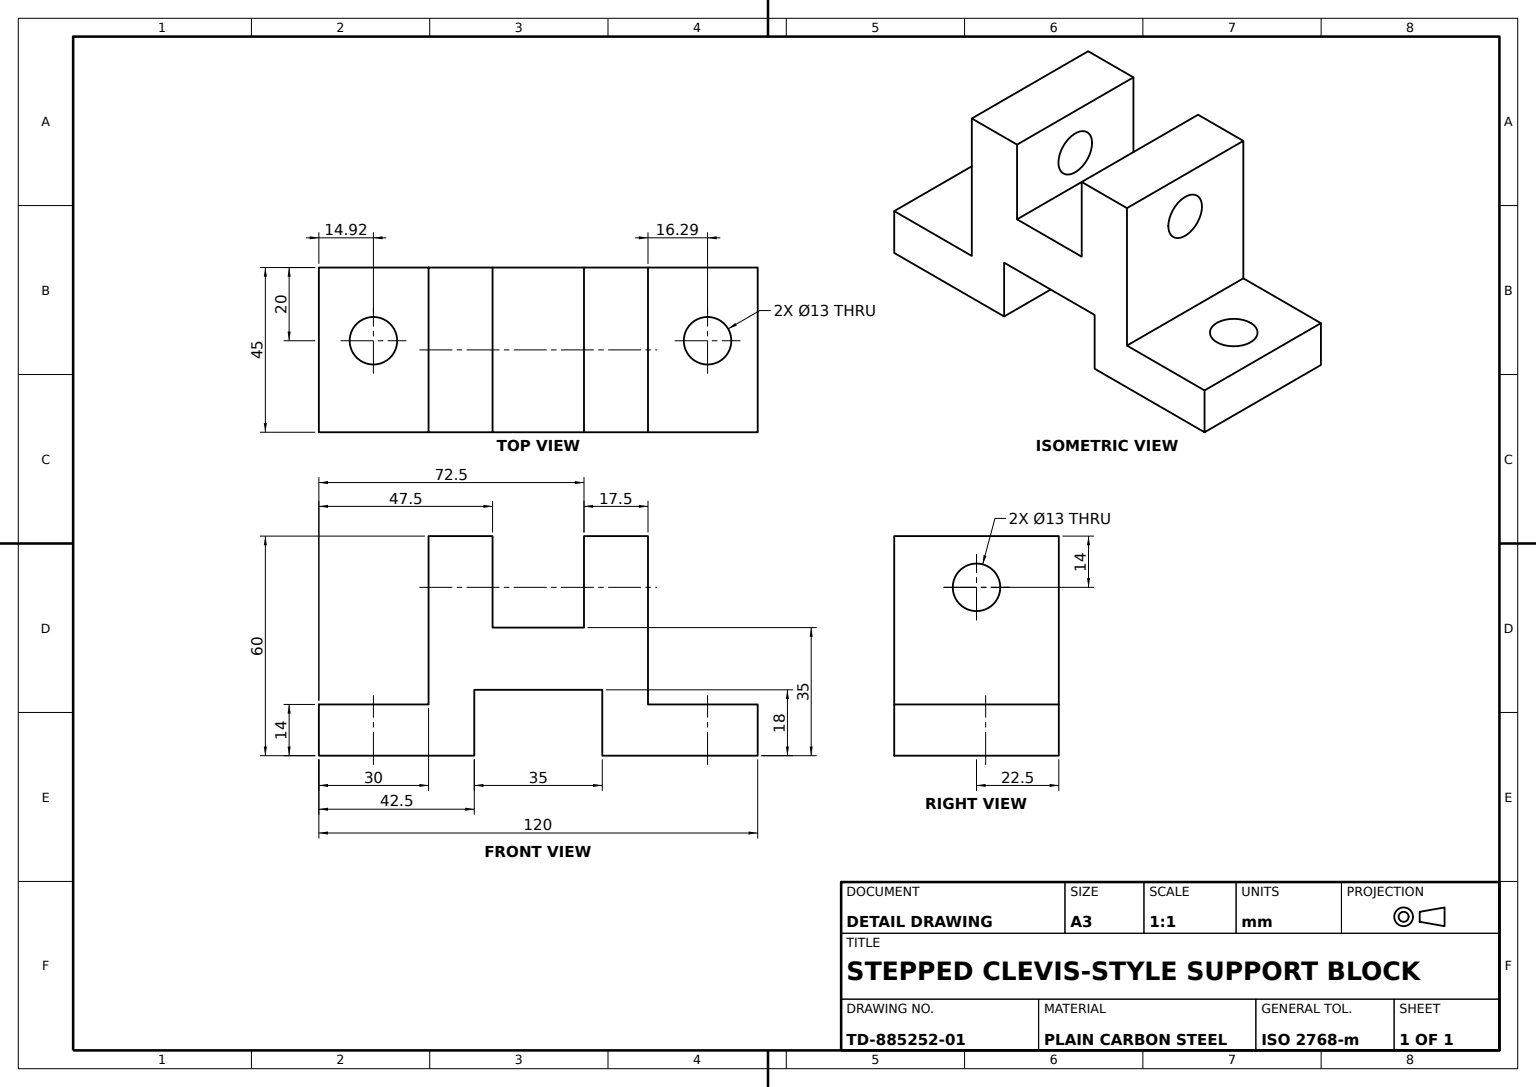
from build123d import *

# Parameters (mm, degrees)
BRACKET_BODY_DEPTH      = 45
UPRIGHT_HOLE_A_SKETCH_R = 6.5
UPRIGHT_HOLE_A_13_DEPTH = 17.5
UPRIGHT_START           = -17.5
UPRIGHT_HOLE_B_SKETCH_R = 6.5
UPRIGHT_HOLE_B_13_DEPTH = 17.5
FLANGE_HOLE_A_SKETCH_R  = 6.5
FLANGE_HOLE_A_13_DEPTH  = 14
FLANGE_HOLE_B_SKETCH_R  = 6.5
FLANGE_HOLE_B_13_DEPTH  = 14


with BuildPart() as part:
    # Bracket Profile Sketch → Bracket Body (new body)
    with BuildSketch(Plane.XY):
        Polygon((0, 0), (42.5, 0), (42.5, 18), (77.5, 18), (77.5, 0), (120, 0), (120, 14), (90, 14), (90, 60), (72.5, 60), (72.5, 35), (47.5, 35), (47.5, 60), (30, 60), (30, 14), (0, 14), align=None)
    extrude(amount=BRACKET_BODY_DEPTH)

    # Upright Hole A Sketch → Upright Hole A Ø13 (cut)
    with BuildSketch(Plane.ZY.offset(-30)):
        with Locations((22.5, 46)):
            Circle(UPRIGHT_HOLE_A_SKETCH_R)
    extrude(amount=-UPRIGHT_HOLE_A_13_DEPTH, mode=Mode.SUBTRACT)

    # Upright Hole B Sketch → Upright Hole B Ø13 (cut)
    with BuildSketch(Plane(origin=(90, 0, 0), x_dir=(0, 0, -1), z_dir=(1, 0, 0)).offset(UPRIGHT_START)):
        with Locations(Location((-22.5, 46, 0), (0, 0, 180))):
            Circle(UPRIGHT_HOLE_B_SKETCH_R)
    extrude(amount=UPRIGHT_HOLE_B_13_DEPTH, mode=Mode.SUBTRACT)

    # Flange Hole A Sketch → Flange Hole A Ø13 (cut)
    with BuildSketch(Plane(origin=(0, 14, 0), x_dir=(1, 0, 0), z_dir=(0, 1, 0))):
        with Locations(Location((14.919656615, -20, 0), (0, 0, 270))):
            Circle(FLANGE_HOLE_A_SKETCH_R)
    extrude(amount=-FLANGE_HOLE_A_13_DEPTH, mode=Mode.SUBTRACT)

    # Flange Hole B Sketch → Flange Hole B Ø13 (cut)
    with BuildSketch(Plane(origin=(0, 14, 0), x_dir=(1, 0, 0), z_dir=(0, 1, 0))):
        with Locations(Location((106.287852583, -20, 0), (0, 0, 270))):
            Circle(FLANGE_HOLE_B_SKETCH_R)
    extrude(amount=-FLANGE_HOLE_B_13_DEPTH, mode=Mode.SUBTRACT)


solid = part.part
